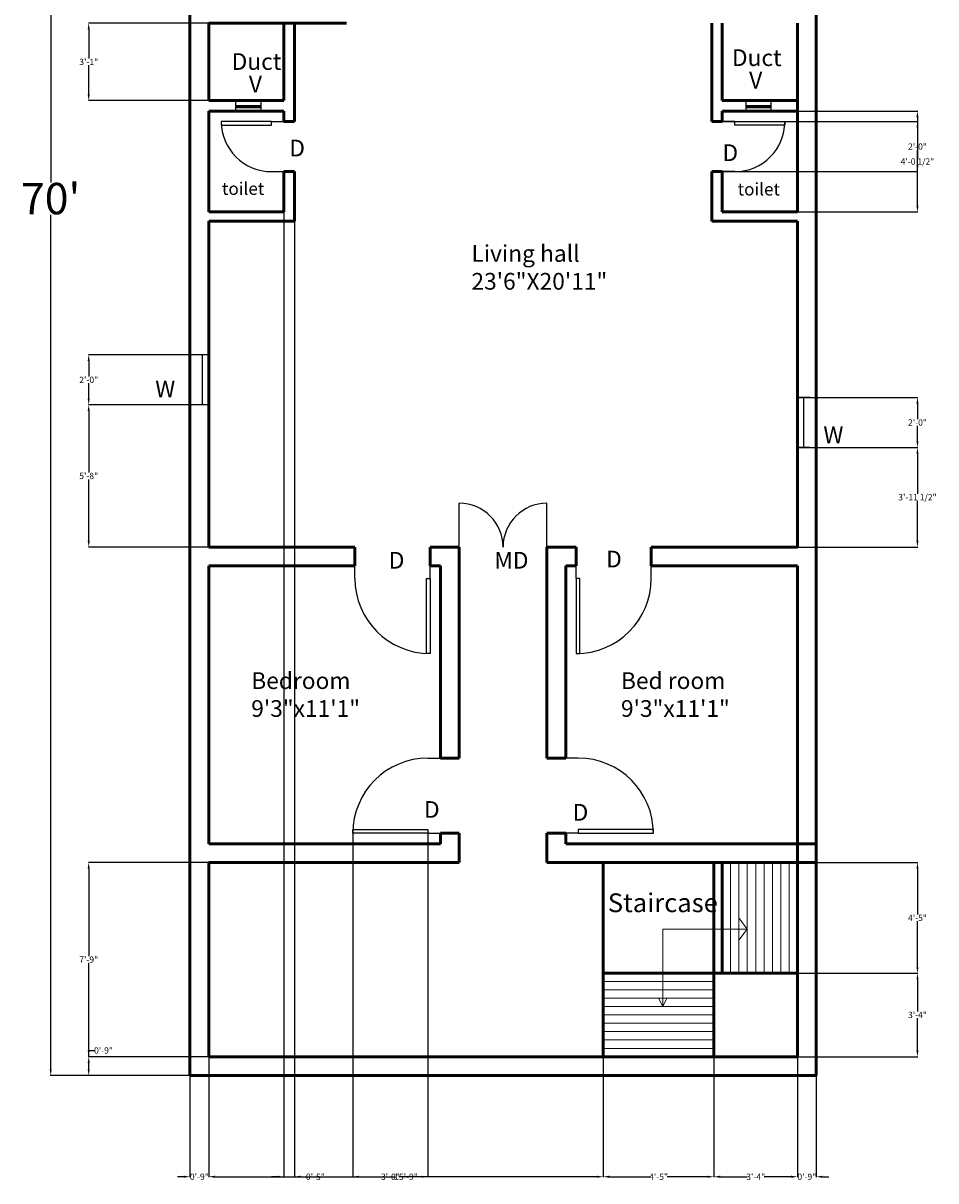
# Model space of a CAD drawing. Units: inches. Extents: x -250 to 2650, y 180 to 1183.
# Tile 9 of 10: x 2212 to 2650, y 180 to 734. Entities that reach past the tile are written whole.
import ezdxf

# ---------------------------------------------------------------- set-up
doc = ezdxf.new("R2010")
doc.units = ezdxf.units.IN
doc.header["$MEASUREMENT"] = 0
for name, color, linetype, lineweight in [('A-ANNO-DIMS', 2, 'Continuous', 18), ('A-ANNO-TEXT', 7, 'Continuous', 18), ('A-AREA-IDEN', 3, 'Continuous', 18), ('A-DOOR', 4, 'Continuous', 25), ('A-FLOR-STRS', 8, 'Continuous', 18), ('A-GLAZ', 3, 'Continuous', 25), ('A-WALL', 7, 'Continuous', 50)]:
    doc.layers.add(name, color=color, linetype=linetype, lineweight=lineweight)
doc.styles.get("Standard").update_dxf_attribs({"font": 'arial.ttf'})
doc.dimstyles.get("Standard").update_dxf_attribs({"dimtxt": 3, "dimasz": 3, "dimexe": 0.18, "dimexo": 0.0625, "dimgap": 0.09, "dimtad": 0, "dimtih": 1, "dimtoh": 1, "dimdec": 0, "dimzin": 0, "dimdsep": 46, "dimlunit": 3, "dimtxsty": 'Standard', "dimcen": 0.09, "dimadec": 0, "dimazin": 0, "dimtfac": 1, "dimtdec": 0, "dimtofl": 0, "dimtmove": 0, "dimatfit": 3, "dimfxl": 1, "dimtolj": 1, "dimtzin": 0, "dimarcsym": 0})

# ---------------------------------------------------------------- blocks, each defined once
blk = doc.blocks.new('*D39')
at = {"layer": 'A-ANNO-DIMS', "color": 0, "lineweight": -2, "transparency": 16777216}
for p, q in [((2292.12, 1070.02), (2225.3, 1070.02)), ((2225.48, 1067.02), (2225.48, 657.77)), ((2225.48, 233.02), (2225.48, 642.28)), ((2292.12, 230.02), (2225.3, 230.02))]:
    blk.add_line(p, q, dxfattribs=at)
at = {"layer": 'A-ANNO-DIMS', "color": 0, "transparency": 16777216}
for points in [[(2224.98, 1067.02), (2225.98, 1067.02), (2225.48, 1070.02)], [(2224.98, 233.02), (2225.98, 233.02), (2225.48, 230.02)]]:
    blk.add_solid(points, dxfattribs=at)
at = {"layer": 'Defpoints', "color": 0, "transparency": 16777216}
for p in [(2292.19, 1070.02), (2225.48, 230.02), (2292.19, 230.02)]:
    blk.add_point(p, dxfattribs=at)
at = {"layer": 'A-ANNO-DIMS', "color": 0, "transparency": 16777216, "insert": (2225.48, 650.02), "char_height": 3, "attachment_point": 5}
blk.add_mtext("\\A1;{\\H5x;70'}", dxfattribs=at)
blk = doc.blocks.new('*U27')
for p, q in [((0, 0), (0, -6)), ((24, 0), (24, -6))]:
    blk.add_line(p, q)
blk.add_lwpolyline([(0, 0), (0, 24), (1.75, 24), (1.75, 0)], close=True)
blk.add_arc((0, 0), 24, 0, 90)
blk = doc.blocks.new('*U28')
for p, q in [((0, 0), (0, 6)), ((24, 0), (24, 6))]:
    blk.add_line(p, q)
blk.add_lwpolyline([(0, 0), (0, -24), (1.75, -24), (1.75, 0)], close=True)
blk.add_arc((0, 0), 24, 270, 0)
blk = doc.blocks.new('*U29')
for p, q in [((0, 5), (0, 0)), ((0, 2.5), (12, 2.5)), ((12, 5), (12, 0))]:
    blk.add_line(p, q)
blk = doc.blocks.new('*U30')
for p, q in [((-36, 0), (-36, -6)), ((0, 0), (0, -6))]:
    blk.add_line(p, q)
blk.add_lwpolyline([(0, 0), (0, 36), (-1.75, 36), (-1.75, 0)], close=True)
blk.add_arc((0, 0), 36, 90, 180)
blk = doc.blocks.new('*U31')
for p, q in [((-36, 0), (-36, 6)), ((0, 0), (0, 6))]:
    blk.add_line(p, q)
blk.add_lwpolyline([(0, 0), (0, -36), (-1.75, -36), (-1.75, 0)], close=True)
blk.add_arc((0, 0), 36, 180, 270)
blk = doc.blocks.new('*U32')
for p, q in [((0, 0), (0, -6)), ((36, 0), (36, -6))]:
    blk.add_line(p, q)
blk.add_lwpolyline([(0, 0), (0, 36), (1.75, 36), (1.75, 0)], close=True)
blk.add_arc((0, 0), 36, 0, 90)
blk = doc.blocks.new('*U33')
for p, q in [((-36, 0), (-36, -6)), ((0, 0), (0, -6))]:
    blk.add_line(p, q)
blk.add_lwpolyline([(0, 0), (0, 36), (-1.75, 36), (-1.75, 0)], close=True)
blk.add_arc((0, 0), 36, 90, 180)
blk = doc.blocks.new('*U23')
for p, q in [((-24, 6), (-24, 0)), ((0, 6), (0, 0)), ((0, 3), (-24, 3))]:
    blk.add_line(p, q)
blk = doc.blocks.new('*U24')
for p, q in [((-24, 6), (-24, 0)), ((0, 6), (0, 0)), ((0, 3), (-24, 3))]:
    blk.add_line(p, q)
blk = doc.blocks.new('DOOR-DOUBLE-MAIN')
for p, q in [((505.08, 483.11), (505.08, 504.11)), ((505.08, 483.11), (505.08, 504.11)), ((547.08, 483.11), (547.08, 504.11))]:
    blk.add_line(p, q)
for centre, start, end in [((505.08, 483.11), 0, 90), ((505.08, 483.11), 0, 90), ((547.08, 483.11), 90, 180)]:
    blk.add_arc(centre, 21, start, end)
blk = doc.blocks.new('*D166')
at = {"layer": 'A-ANNO-DIMS', "color": 0, "lineweight": -2, "transparency": 16777216}
for p, q in [((2583.185258, 238.962048), (2583.185258, 181.344548)), ((2592.185258, 229.962048), (2592.185258, 181.344548)), ((2580.185258, 181.524548), (2577.185258, 181.524548)), ((2595.185258, 181.524548), (2598.185258, 181.524548))]:
    blk.add_line(p, q, dxfattribs=at)
at = {"layer": 'A-ANNO-DIMS', "color": 0, "transparency": 16777216}
for points in [[(2580.185258, 182.024548), (2580.185258, 181.024548), (2583.185258, 181.524548)], [(2595.185258, 182.024548), (2595.185258, 181.024548), (2592.185258, 181.524548)]]:
    blk.add_solid(points, dxfattribs=at)
at = {"layer": 'Defpoints', "color": 0, "transparency": 16777216}
for p in [(2583.185258, 239.024548), (2592.185258, 230.024548), (2592.185258, 181.524548)]:
    blk.add_point(p, dxfattribs=at)
at = {"layer": 'A-ANNO-DIMS', "color": 0, "transparency": 16777216, "insert": (2587.685258, 181.524548), "char_height": 3, "attachment_point": 5}
blk.add_mtext('\\A1;0\'-9"', dxfattribs=at)
blk = doc.blocks.new('*D167')
at = {"layer": 'A-ANNO-DIMS', "color": 0, "lineweight": -2, "transparency": 16777216}
for p, q in [((2301.185258, 238.962048), (2301.185258, 181.344548)), ((2292.185258, 229.962048), (2292.185258, 181.344548)), ((2289.185258, 181.524548), (2286.185258, 181.524548)), ((2304.185258, 181.524548), (2307.185258, 181.524548))]:
    blk.add_line(p, q, dxfattribs=at)
at = {"layer": 'A-ANNO-DIMS', "color": 0, "transparency": 16777216}
for points in [[(2289.185258, 182.024548), (2289.185258, 181.024548), (2292.185258, 181.524548)], [(2304.185258, 182.024548), (2304.185258, 181.024548), (2301.185258, 181.524548)]]:
    blk.add_solid(points, dxfattribs=at)
at = {"layer": 'Defpoints', "color": 0, "transparency": 16777216}
for p in [(2301.185258, 239.024548), (2292.185258, 230.024548), (2301.185258, 181.524548)]:
    blk.add_point(p, dxfattribs=at)
at = {"layer": 'A-ANNO-DIMS', "color": 0, "transparency": 16777216, "insert": (2296.685258, 181.524548), "char_height": 3, "attachment_point": 5}
blk.add_mtext('\\A1;0\'-9"', dxfattribs=at)
blk = doc.blocks.new('*D168')
at = {"layer": 'A-ANNO-DIMS', "color": 0, "lineweight": -2, "transparency": 16777216}
for p, q in [((2301.19, 238.96), (2301.19, 181.34)), ((2490.19, 238.96), (2490.19, 181.34)), ((2304.19, 181.52), (2390.58, 181.52)), ((2487.19, 181.52), (2400.79, 181.52))]:
    blk.add_line(p, q, dxfattribs=at)
at = {"layer": 'A-ANNO-DIMS', "color": 0, "transparency": 16777216}
for points in [[(2304.19, 182.02), (2304.19, 181.02), (2301.19, 181.52)], [(2487.19, 182.02), (2487.19, 181.02), (2490.19, 181.52)]]:
    blk.add_solid(points, dxfattribs=at)
at = {"layer": 'Defpoints', "color": 0, "transparency": 16777216}
for p in [(2301.19, 239.02), (2490.19, 239.02), (2490.19, 181.52)]:
    blk.add_point(p, dxfattribs=at)
at = {"layer": 'A-ANNO-DIMS', "color": 0, "transparency": 16777216, "insert": (2395.69, 181.52), "char_height": 3, "attachment_point": 5}
blk.add_mtext('\\A1;15\'-9"', dxfattribs=at)
blk = doc.blocks.new('*D169')
at = {"layer": 'A-ANNO-DIMS', "color": 0, "lineweight": -2, "transparency": 16777216}
for p, q in [((2490.19, 238.96), (2490.19, 181.34)), ((2543.19, 238.96), (2543.19, 181.34)), ((2493.19, 181.52), (2512.55, 181.52)), ((2540.19, 181.52), (2520.82, 181.52))]:
    blk.add_line(p, q, dxfattribs=at)
at = {"layer": 'A-ANNO-DIMS', "color": 0, "transparency": 16777216}
for points in [[(2493.19, 182.02), (2493.19, 181.02), (2490.19, 181.52)], [(2540.19, 182.02), (2540.19, 181.02), (2543.19, 181.52)]]:
    blk.add_solid(points, dxfattribs=at)
at = {"layer": 'Defpoints', "color": 0, "transparency": 16777216}
for p in [(2490.19, 239.02), (2543.19, 239.02), (2543.19, 181.52)]:
    blk.add_point(p, dxfattribs=at)
at = {"layer": 'A-ANNO-DIMS', "color": 0, "transparency": 16777216, "insert": (2516.69, 181.52), "char_height": 3, "attachment_point": 5}
blk.add_mtext('\\A1;4\'-5"', dxfattribs=at)
blk = doc.blocks.new('*D170')
at = {"layer": 'A-ANNO-DIMS', "color": 0, "lineweight": -2, "transparency": 16777216}
for p, q in [((2543.19, 238.96), (2543.19, 181.34)), ((2583.19, 238.96), (2583.19, 181.34)), ((2546.19, 181.52), (2559.11, 181.52)), ((2580.19, 181.52), (2567.26, 181.52))]:
    blk.add_line(p, q, dxfattribs=at)
at = {"layer": 'A-ANNO-DIMS', "color": 0, "transparency": 16777216}
for points in [[(2546.19, 182.02), (2546.19, 181.02), (2543.19, 181.52)], [(2580.19, 182.02), (2580.19, 181.02), (2583.19, 181.52)]]:
    blk.add_solid(points, dxfattribs=at)
at = {"layer": 'Defpoints', "color": 0, "transparency": 16777216}
for p in [(2543.19, 239.02), (2583.19, 239.02), (2583.19, 181.52)]:
    blk.add_point(p, dxfattribs=at)
at = {"layer": 'A-ANNO-DIMS', "color": 0, "transparency": 16777216, "insert": (2563.19, 181.52), "char_height": 3, "attachment_point": 5}
blk.add_mtext('\\A1;3\'-4"', dxfattribs=at)
blk = doc.blocks.new('*D171')
at = {"layer": 'A-ANNO-DIMS', "color": 0, "lineweight": -2, "transparency": 16777216}
for p, q in [((2583.25, 279.02), (2640.87, 279.02)), ((2640.69, 276.02), (2640.69, 260.65)), ((2640.69, 242.02), (2640.69, 257.4)), ((2583.25, 239.02), (2640.87, 239.02))]:
    blk.add_line(p, q, dxfattribs=at)
at = {"layer": 'A-ANNO-DIMS', "color": 0, "transparency": 16777216}
for points in [[(2640.19, 276.02), (2641.19, 276.02), (2640.69, 279.02)], [(2640.19, 242.02), (2641.19, 242.02), (2640.69, 239.02)]]:
    blk.add_solid(points, dxfattribs=at)
at = {"layer": 'Defpoints', "color": 0, "transparency": 16777216}
for p in [(2583.19, 279.02), (2640.69, 279.02), (2583.19, 239.02)]:
    blk.add_point(p, dxfattribs=at)
at = {"layer": 'A-ANNO-DIMS', "color": 0, "transparency": 16777216, "insert": (2640.69, 259.02), "char_height": 3, "attachment_point": 5}
blk.add_mtext('\\A1;3\'-4"', dxfattribs=at)
blk = doc.blocks.new('*D172')
at = {"layer": 'A-ANNO-DIMS', "color": 0, "lineweight": -2, "transparency": 16777216}
for p, q in [((2579.25, 332.02), (2640.87, 332.02)), ((2640.69, 329.02), (2640.69, 307.14)), ((2640.69, 282.02), (2640.69, 303.91)), ((2583.25, 279.02), (2640.87, 279.02))]:
    blk.add_line(p, q, dxfattribs=at)
at = {"layer": 'A-ANNO-DIMS', "color": 0, "transparency": 16777216}
for points in [[(2640.19, 329.02), (2641.19, 329.02), (2640.69, 332.02)], [(2640.19, 282.02), (2641.19, 282.02), (2640.69, 279.02)]]:
    blk.add_solid(points, dxfattribs=at)
at = {"layer": 'Defpoints', "color": 0, "transparency": 16777216}
for p in [(2579.19, 332.02), (2640.69, 332.02), (2583.19, 279.02)]:
    blk.add_point(p, dxfattribs=at)
at = {"layer": 'A-ANNO-DIMS', "color": 0, "transparency": 16777216, "insert": (2640.69, 305.52), "char_height": 3, "attachment_point": 5}
blk.add_mtext('\\A1;4\'-5"', dxfattribs=at)
blk = doc.blocks.new('*D173')
at = {"layer": 'A-ANNO-DIMS', "color": 0, "lineweight": -2, "transparency": 16777216}
for p, q in [((2301.12, 239.02), (2243.51, 239.02)), ((2243.69, 239.02), (2243.69, 242.02)), ((2243.69, 242.02), (2246.69, 242.02)), ((2243.69, 233.02), (2243.69, 236.02)), ((2292.12, 230.02), (2243.51, 230.02))]:
    blk.add_line(p, q, dxfattribs=at)
at = {"layer": 'A-ANNO-DIMS', "color": 0, "transparency": 16777216}
for points in [[(2243.19, 236.02), (2244.19, 236.02), (2243.69, 239.02)], [(2243.19, 233.02), (2244.19, 233.02), (2243.69, 230.02)]]:
    blk.add_solid(points, dxfattribs=at)
at = {"layer": 'Defpoints', "color": 0, "transparency": 16777216}
for p in [(2243.69, 239.02), (2301.19, 239.02), (2292.19, 230.02)]:
    blk.add_point(p, dxfattribs=at)
at = {"layer": 'A-ANNO-DIMS', "color": 0, "transparency": 16777216, "insert": (2250.76, 242.02), "char_height": 3, "attachment_point": 5}
blk.add_mtext('\\A1;0\'-9"', dxfattribs=at)
blk = doc.blocks.new('*D174')
at = {"layer": 'A-ANNO-DIMS', "color": 0, "lineweight": -2, "transparency": 16777216}
for p, q in [((2301.12, 332.02), (2243.51, 332.02)), ((2243.69, 329.02), (2243.69, 287.15)), ((2243.69, 242.02), (2243.69, 283.9)), ((2301.12, 239.02), (2243.51, 239.02))]:
    blk.add_line(p, q, dxfattribs=at)
at = {"layer": 'A-ANNO-DIMS', "color": 0, "transparency": 16777216}
for points in [[(2243.19, 329.02), (2244.19, 329.02), (2243.69, 332.02)], [(2243.19, 242.02), (2244.19, 242.02), (2243.69, 239.02)]]:
    blk.add_solid(points, dxfattribs=at)
at = {"layer": 'Defpoints', "color": 0, "transparency": 16777216}
for p in [(2243.69, 332.02), (2301.19, 332.02), (2301.19, 239.02)]:
    blk.add_point(p, dxfattribs=at)
at = {"layer": 'A-ANNO-DIMS', "color": 0, "transparency": 16777216, "insert": (2243.69, 285.52), "char_height": 3, "attachment_point": 5}
blk.add_mtext('\\A1;7\'-9"', dxfattribs=at)
blk = doc.blocks.new('*D176')
at = {"layer": 'A-ANNO-DIMS', "color": 0, "lineweight": -2, "transparency": 16777216}
for p, q in [((2337.19, 643.56), (2337.19, 181.34)), ((2342.19, 639.05), (2342.19, 181.34)), ((2334.19, 181.52), (2331.19, 181.52)), ((2345.19, 181.52), (2348.19, 181.52))]:
    blk.add_line(p, q, dxfattribs=at)
at = {"layer": 'A-ANNO-DIMS', "color": 0, "transparency": 16777216}
for points in [[(2334.19, 182.02), (2334.19, 181.02), (2337.19, 181.52)], [(2345.19, 182.02), (2345.19, 181.02), (2342.19, 181.52)]]:
    blk.add_solid(points, dxfattribs=at)
at = {"layer": 'Defpoints', "color": 0, "transparency": 16777216}
for p in [(2337.19, 643.62), (2342.19, 639.11), (2342.19, 181.52)]:
    blk.add_point(p, dxfattribs=at)
at = {"layer": 'A-ANNO-DIMS', "color": 0, "transparency": 16777216, "insert": (2352.26, 181.52), "char_height": 3, "attachment_point": 5}
blk.add_mtext('\\A1;0\'-5"', dxfattribs=at)
blk = doc.blocks.new('*D177')
at = {"layer": 'A-ANNO-DIMS', "color": 0, "lineweight": -2, "transparency": 16777216}
for p, q in [((2301.12, 734.02), (2243.51, 734.02)), ((2243.69, 731.02), (2243.69, 717.09)), ((2243.69, 699.91), (2243.69, 713.84)), ((2301.12, 696.91), (2243.51, 696.91))]:
    blk.add_line(p, q, dxfattribs=at)
at = {"layer": 'A-ANNO-DIMS', "color": 0, "transparency": 16777216}
for points in [[(2243.19, 731.02), (2244.19, 731.02), (2243.69, 734.02)], [(2243.19, 699.91), (2244.19, 699.91), (2243.69, 696.91)]]:
    blk.add_solid(points, dxfattribs=at)
at = {"layer": 'Defpoints', "color": 0, "transparency": 16777216}
for p in [(2243.69, 734.02), (2301.19, 734.02), (2301.19, 696.91)]:
    blk.add_point(p, dxfattribs=at)
at = {"layer": 'A-ANNO-DIMS', "color": 0, "transparency": 16777216, "insert": (2243.69, 715.47), "char_height": 3, "attachment_point": 5}
blk.add_mtext('\\A1;3\'-1"', dxfattribs=at)
blk = doc.blocks.new('*D178')
at = {"layer": 'A-ANNO-DIMS', "color": 0, "lineweight": -2, "transparency": 16777216}
for p, q in [((2583.25, 691.91), (2640.87, 691.91)), ((2640.69, 688.91), (2640.69, 669.41)), ((2640.69, 646.62), (2640.69, 666.12)), ((2583.25, 643.62), (2640.87, 643.62))]:
    blk.add_line(p, q, dxfattribs=at)
at = {"layer": 'A-ANNO-DIMS', "color": 0, "transparency": 16777216}
for points in [[(2640.19, 688.91), (2641.19, 688.91), (2640.69, 691.91)], [(2640.19, 646.62), (2641.19, 646.62), (2640.69, 643.62)]]:
    blk.add_solid(points, dxfattribs=at)
at = {"layer": 'Defpoints', "color": 0, "transparency": 16777216}
for p in [(2583.19, 691.91), (2640.69, 691.91), (2583.19, 643.62)]:
    blk.add_point(p, dxfattribs=at)
at = {"layer": 'A-ANNO-DIMS', "color": 0, "transparency": 16777216, "insert": (2640.69, 667.77), "char_height": 3, "attachment_point": 5}
blk.add_mtext('\\A1;4\'-0 1/2"', dxfattribs=at)
blk = doc.blocks.new('*D179')
at = {"layer": 'A-ANNO-DIMS', "color": 0, "lineweight": -2, "transparency": 16777216}
for p, q in [((2583.25, 530.79), (2640.87, 530.79)), ((2640.69, 527.79), (2640.69, 508.59)), ((2640.69, 486.11), (2640.69, 505.31)), ((2583.25, 483.11), (2640.87, 483.11))]:
    blk.add_line(p, q, dxfattribs=at)
at = {"layer": 'A-ANNO-DIMS', "color": 0, "transparency": 16777216}
for points in [[(2640.19, 527.79), (2641.19, 527.79), (2640.69, 530.79)], [(2640.19, 486.11), (2641.19, 486.11), (2640.69, 483.11)]]:
    blk.add_solid(points, dxfattribs=at)
at = {"layer": 'Defpoints', "color": 0, "transparency": 16777216}
for p in [(2583.19, 530.79), (2640.69, 530.79), (2583.19, 483.11)]:
    blk.add_point(p, dxfattribs=at)
at = {"layer": 'A-ANNO-DIMS', "color": 0, "transparency": 16777216, "insert": (2640.69, 506.95), "char_height": 3, "attachment_point": 5}
blk.add_mtext('\\A1;3\'-11 1/2"', dxfattribs=at)
blk = doc.blocks.new('*D180')
at = {"layer": 'A-ANNO-DIMS', "color": 0, "lineweight": -2, "transparency": 16777216}
for p, q in [((2583.25, 554.79), (2640.87, 554.79)), ((2640.69, 551.79), (2640.69, 544.41)), ((2640.69, 533.79), (2640.69, 541.16)), ((2583.25, 530.79), (2640.87, 530.79))]:
    blk.add_line(p, q, dxfattribs=at)
at = {"layer": 'A-ANNO-DIMS', "color": 0, "transparency": 16777216}
for points in [[(2640.19, 551.79), (2641.19, 551.79), (2640.69, 554.79)], [(2640.19, 533.79), (2641.19, 533.79), (2640.69, 530.79)]]:
    blk.add_solid(points, dxfattribs=at)
at = {"layer": 'Defpoints', "color": 0, "transparency": 16777216}
for p in [(2583.19, 554.79), (2640.69, 554.79), (2583.19, 530.79)]:
    blk.add_point(p, dxfattribs=at)
at = {"layer": 'A-ANNO-DIMS', "color": 0, "transparency": 16777216, "insert": (2640.69, 542.79), "char_height": 3, "attachment_point": 5}
blk.add_mtext('\\A1;2\'-0"', dxfattribs=at)
blk = doc.blocks.new('*D181')
at = {"layer": 'A-ANNO-DIMS', "color": 0, "lineweight": -2, "transparency": 16777216}
for p, q in [((2301.12, 551.2), (2243.51, 551.2)), ((2243.69, 548.2), (2243.69, 518.78)), ((2243.69, 486.11), (2243.69, 515.53)), ((2301.12, 483.11), (2243.51, 483.11))]:
    blk.add_line(p, q, dxfattribs=at)
at = {"layer": 'A-ANNO-DIMS', "color": 0, "transparency": 16777216}
for points in [[(2243.19, 548.2), (2244.19, 548.2), (2243.69, 551.2)], [(2243.19, 486.11), (2244.19, 486.11), (2243.69, 483.11)]]:
    blk.add_solid(points, dxfattribs=at)
at = {"layer": 'Defpoints', "color": 0, "transparency": 16777216}
for p in [(2243.69, 551.2), (2301.19, 551.2), (2301.19, 483.11)]:
    blk.add_point(p, dxfattribs=at)
at = {"layer": 'A-ANNO-DIMS', "color": 0, "transparency": 16777216, "insert": (2243.69, 517.16), "char_height": 3, "attachment_point": 5}
blk.add_mtext('\\A1;5\'-8"', dxfattribs=at)
blk = doc.blocks.new('*D182')
at = {"layer": 'A-ANNO-DIMS', "color": 0, "lineweight": -2, "transparency": 16777216}
for p, q in [((2301.12, 575.2), (2243.51, 575.2)), ((2243.69, 572.2), (2243.69, 564.82)), ((2243.69, 554.2), (2243.69, 561.58)), ((2301.12, 551.2), (2243.51, 551.2))]:
    blk.add_line(p, q, dxfattribs=at)
at = {"layer": 'A-ANNO-DIMS', "color": 0, "transparency": 16777216}
for points in [[(2243.19, 572.2), (2244.19, 572.2), (2243.69, 575.2)], [(2243.19, 554.2), (2244.19, 554.2), (2243.69, 551.2)]]:
    blk.add_solid(points, dxfattribs=at)
at = {"layer": 'Defpoints', "color": 0, "transparency": 16777216}
for p in [(2243.69, 575.2), (2301.19, 575.2), (2301.19, 551.2)]:
    blk.add_point(p, dxfattribs=at)
at = {"layer": 'A-ANNO-DIMS', "color": 0, "transparency": 16777216, "insert": (2243.69, 563.2), "char_height": 3, "attachment_point": 5}
blk.add_mtext('\\A1;2\'-0"', dxfattribs=at)
blk = doc.blocks.new('*D183')
at = {"layer": 'A-ANNO-DIMS', "color": 0, "lineweight": -2, "transparency": 16777216}
for p, q in [((2370.19, 345.96), (2370.19, 181.34)), ((2406.19, 345.96), (2406.19, 181.34)), ((2373.19, 181.52), (2384.11, 181.52)), ((2403.19, 181.52), (2392.26, 181.52))]:
    blk.add_line(p, q, dxfattribs=at)
at = {"layer": 'A-ANNO-DIMS', "color": 0, "transparency": 16777216}
for points in [[(2373.19, 182.02), (2373.19, 181.02), (2370.19, 181.52)], [(2403.19, 182.02), (2403.19, 181.02), (2406.19, 181.52)]]:
    blk.add_solid(points, dxfattribs=at)
at = {"layer": 'Defpoints', "color": 0, "transparency": 16777216}
for p in [(2370.19, 346.02), (2406.19, 346.02), (2406.19, 181.52)]:
    blk.add_point(p, dxfattribs=at)
at = {"layer": 'A-ANNO-DIMS', "color": 0, "transparency": 16777216, "insert": (2388.19, 181.52), "char_height": 3, "attachment_point": 5}
blk.add_mtext('\\A1;3\'-0"', dxfattribs=at)
blk = doc.blocks.new('*D184')
at = {"layer": 'A-ANNO-DIMS', "color": 0, "lineweight": -2, "transparency": 16777216}
for p, q in [((2542.25, 686.91), (2640.87, 686.91)), ((2640.69, 683.91), (2640.69, 676.53)), ((2640.69, 665.91), (2640.69, 673.29)), ((2542.25, 662.91), (2640.87, 662.91))]:
    blk.add_line(p, q, dxfattribs=at)
at = {"layer": 'A-ANNO-DIMS', "color": 0, "transparency": 16777216}
for points in [[(2640.19, 683.91), (2641.19, 683.91), (2640.69, 686.91)], [(2640.19, 665.91), (2641.19, 665.91), (2640.69, 662.91)]]:
    blk.add_solid(points, dxfattribs=at)
at = {"layer": 'Defpoints', "color": 0, "transparency": 16777216}
for p in [(2542.19, 686.91), (2640.69, 686.91), (2542.19, 662.91)]:
    blk.add_point(p, dxfattribs=at)
at = {"layer": 'A-ANNO-DIMS', "color": 0, "transparency": 16777216, "insert": (2640.69, 674.91), "char_height": 3, "attachment_point": 5}
blk.add_mtext('\\A1;2\'-0"', dxfattribs=at)

msp = doc.modelspace()

# ---------------------------------------------------------------- linework, layer by layer
at = {"layer": 'A-FLOR-STRS'}
for p, q in [((2551.19, 279.02), (2551.19, 332.02)), ((2555.19, 279.02), (2555.19, 332.02)), ((2559.19, 279.02), (2559.19, 332.02)), ((2563.19, 279.02), (2563.19, 332.02)), ((2567.19, 279.02), (2567.19, 332.02)), ((2571.19, 279.02), (2571.19, 332.02)), ((2575.19, 279.02), (2575.19, 332.02)), ((2579.19, 279.02), (2579.19, 332.02)), ((2559.19, 300.14), (2555.19, 305.52)), ((2518.7, 300.14), (2518.7, 263.02)), ((2518.7, 300.14), (2559.19, 300.14)), ((2559.19, 300.14), (2555.19, 294.75)), ((2490.19, 275.02), (2543.19, 275.02)), ((2490.19, 271.02), (2543.19, 271.02)), ((2490.19, 267.02), (2543.19, 267.02)), ((2518.7, 263.02), (2516.69, 267.02)), ((2518.7, 263.02), (2520.71, 267.02)), ((2490.19, 263.02), (2543.19, 263.02)), ((2490.19, 259.02), (2543.19, 259.02)), ((2490.19, 255.02), (2543.19, 255.02)), ((2490.19, 251.02), (2543.19, 251.02)), ((2490.19, 247.02), (2543.19, 247.02)), ((2490.19, 243.02), (2543.19, 243.02))]:
    msp.add_line(p, q, dxfattribs=at)
at = {"layer": 'A-WALL'}
for p, q in [((2292.19, 1070.02), (2292.19, 230.02)), ((2592.19, 230.02), (2592.19, 1070.02)), ((2367.19, 734.02), (2301.19, 734.02)), ((2301.19, 734.02), (2301.19, 696.91)), ((2337.19, 696.91), (2337.19, 734.02)), ((2342.19, 686.91), (2342.19, 734.02)), ((2542.19, 686.91), (2542.19, 734.02)), ((2542.19, 686.91), (2542.19, 734.02)), ((2547.19, 696.91), (2547.19, 734.02)), ((2583.19, 643.62), (2583.19, 734.02)), ((2583.19, 696.91), (2583.19, 734.02)), ((2583.19, 716.02), (2583.19, 734.02)), ((2337.19, 696.91), (2301.19, 696.91)), ((2326.24, 693.93), (2314.24, 693.93)), ((2583.19, 696.91), (2547.19, 696.91)), ((2570.63, 693.93), (2558.63, 693.93)), ((2301.19, 691.91), (2301.19, 643.62)), ((2337.19, 691.91), (2301.19, 691.91)), ((2337.19, 691.91), (2337.19, 686.91)), ((2547.19, 686.91), (2547.19, 691.91)), ((2583.19, 691.91), (2547.19, 691.91)), ((2583.19, 643.62), (2583.19, 691.91)), ((2337.19, 686.91), (2342.19, 686.91)), ((2547.19, 686.91), (2542.19, 686.91)), ((2337.19, 662.91), (2337.19, 643.62)), ((2337.19, 662.91), (2342.19, 662.91)), ((2342.19, 639.11), (2342.19, 662.91)), ((2342.19, 662.91), (2342.19, 639.11)), ((2542.19, 639.11), (2542.19, 662.91)), ((2542.19, 643.62), (2542.19, 662.91)), ((2547.19, 662.91), (2542.19, 662.91)), ((2547.19, 643.62), (2547.19, 662.91)), ((2337.19, 643.62), (2301.19, 643.62)), ((2342.19, 643.62), (2342.19, 643.62)), ((2583.19, 643.62), (2547.19, 643.62)), ((2301.19, 639.11), (2301.19, 483.11)), ((2342.19, 639.11), (2301.19, 639.11)), ((2583.19, 639.11), (2542.19, 639.11)), ((2583.19, 483.11), (2583.19, 639.11)), ((2583.19, 587.02), (2583.19, 639.11)), ((2371.19, 483.11), (2301.19, 483.11)), ((2371.19, 474.11), (2371.19, 483.11)), ((2421.19, 483.11), (2407.19, 483.11)), ((2407.19, 474.11), (2407.19, 483.11)), ((2421.19, 483.11), (2421.19, 382.02)), ((2463.19, 382.02), (2463.19, 483.11)), ((2477.19, 483.11), (2463.19, 483.11)), ((2477.19, 474.11), (2477.19, 483.11)), ((2583.19, 483.11), (2513.19, 483.11)), ((2513.19, 474.11), (2513.19, 483.11)), ((2301.19, 474.11), (2301.19, 341.02)), ((2371.19, 474.11), (2301.19, 474.11)), ((2412.19, 474.11), (2407.19, 474.11)), ((2412.19, 474.11), (2412.19, 382.02)), ((2472.19, 382.02), (2472.19, 474.11)), ((2477.19, 474.11), (2472.19, 474.11)), ((2583.19, 474.11), (2513.19, 474.11)), ((2583.19, 239.02), (2583.19, 474.11)), ((2412.19, 382.02), (2421.19, 382.02)), ((2463.19, 382.02), (2472.19, 382.02)), ((2412.19, 346.02), (2412.19, 341.02)), ((2412.19, 346.02), (2421.19, 346.02)), ((2421.19, 346.02), (2421.19, 332.02)), ((2463.19, 332.02), (2463.19, 346.02)), ((2472.19, 346.02), (2463.19, 346.02)), ((2472.19, 341.02), (2472.19, 346.02)), ((2301.19, 341.02), (2412.19, 341.02)), ((2472.19, 341.02), (2592.19, 341.02)), ((2301.19, 332.02), (2421.19, 332.02)), ((2301.19, 332.02), (2301.19, 239.02)), ((2463.19, 332.02), (2592.19, 332.02)), ((2490.19, 239.02), (2490.19, 332.02)), ((2543.19, 239.02), (2543.19, 332.02)), ((2547.19, 279.02), (2547.19, 332.02)), ((2490.19, 279.02), (2583.19, 279.02)), ((2301.19, 239.02), (2325.94, 239.02)), ((2301.19, 239.02), (2583.19, 239.02)), ((2292.19, 230.02), (2325.19, 230.02)), ((2292.19, 230.02), (2592.19, 230.02))]:
    msp.add_line(p, q, dxfattribs=at)

# ---------------------------------------------------------------- block references
at = {"layer": 'A-DOOR'}
for name, p, rotation in [('*U28', (2331.19, 686.91), 270), ('*U27', (2553.19, 686.91), 270), ('*U32', (2407.19, 468.11), 180), ('*U33', (2477.19, 468.11), 180), ('*U31', (2406.19, 346.02), 270), ('*U30', (2478.19, 346.02), 270)]:
    msp.add_blockref(name, p, dxfattribs=dict(at, rotation=rotation))
msp.add_blockref('DOOR-DOUBLE-MAIN', (1916.1, 0), dxfattribs=at)
at = {"layer": 'A-GLAZ'}
for name, p, rotation in [('*U29', (2326.24, 696.91), 180), ('*U29', (2570.63, 696.91), 180), ('*U23', (2295.19, 551.2), 270), ('*U24', (2583.19, 530.79), 270)]:
    msp.add_blockref(name, p, dxfattribs=dict(at, rotation=rotation))

# ---------------------------------------------------------------- texts
at = {"layer": 'A-ANNO-TEXT', "char_height": 8, "attachment_point": 1}
for s, insert in [('V', (2560.06, 710.71)), ('V', (2320.41, 708.86)), ('D', (2339.77, 678.19)), ('D', (2547.27, 675.98)), ('W', (2275.55, 562.85)), ('W', (2595.62, 540.86)), ('D', (2387.42, 480.78)), ('MD', (2437.99, 480.78)), ('D', (2491.54, 481.35)), ('D', (2404.29, 361.42)), ('D', (2475.5, 360.07))]:
    msp.add_mtext_dynamic_manual_height_columns(s, width=10.3916, gutter_width=1, heights=[0], dxfattribs=dict(at, insert=insert))
at = {"layer": 'A-AREA-IDEN', "attachment_point": 1}
for s, width, heights, insert, char_height in [('{\\H2.66667x;Duct} ', 7.71, [3.05], (2551.8, 721.49), 3), ('{\\H2.66667x;Duct} ', 7.71, [3.05], (2312.15, 719.65), 3), ('toilet', 19.3499, [0], (2307.53, 657.78), 6), ('toilet', 19.3499, [0], (2554.57, 657.5), 6), ('Living hall  \\P23\'6"X20\'11"', 123.5412, [0], (2427.03, 627.72), 8), ('Bedroom 9\'3"x11\'1"', 88.0689, [0], (2321.54, 423.12), 8), ('Bed room 9\'3"x11\'1"', 88.0689, [0], (2498.66, 423.12), 8), ('Staircase  ', 87.4783, [0], (2492.36, 317.24), 9)]:
    msp.add_mtext_dynamic_manual_height_columns(s, width=width, gutter_width=1, heights=heights, dxfattribs=dict(at, insert=insert, char_height=char_height))

# ---------------------------------------------------------------- dimensions: what is measured, and where the dimension line sits
at = {"layer": 'A-ANNO-DIMS'}
dim = msp.add_linear_dim(base=(2225.48, 230.02), p1=(2292.19, 1070.02), p2=(2292.19, 230.02), angle=90, text='{\\H5x;<>}', dimstyle='Standard', override={"dimclrd": 0, "dimclre": 0, "dimclrt": 0}, dxfattribs=at)
dim.commit()
dim.dimension.update_dxf_attribs({"geometry": '*D39', "text_midpoint": (2225.48, 650.02)})
for base, p1, p2, picture, middle in [((2243.69, 734.02), (2301.19, 696.91), (2301.19, 734.02), '*D177', (2243.69, 715.47)), ((2640.69, 691.91), (2583.19, 643.62), (2583.19, 691.91), '*D178', (2640.69, 667.77)), ((2640.69, 686.91), (2542.19, 662.91), (2542.19, 686.91), '*D184', (2640.69, 674.91)), ((2243.69, 575.2), (2301.19, 551.2), (2301.19, 575.2), '*D182', (2243.69, 563.2)), ((2640.69, 554.79), (2583.19, 530.79), (2583.19, 554.79), '*D180', (2640.69, 542.79)), ((2243.69, 551.2), (2301.19, 483.11), (2301.19, 551.2), '*D181', (2243.69, 517.16)), ((2640.69, 530.79), (2583.19, 483.11), (2583.19, 530.79), '*D179', (2640.69, 506.95)), ((2243.69, 332.02), (2301.19, 239.02), (2301.19, 332.02), '*D174', (2243.69, 285.52)), ((2640.69, 332.02), (2583.19, 279.02), (2579.19, 332.02), '*D172', (2640.69, 305.52)), ((2640.69, 279.02), (2583.19, 239.02), (2583.19, 279.02), '*D171', (2640.69, 259.02)), ((2243.69, 239.02), (2292.19, 230.02), (2301.19, 239.02), '*D173', (2250.76, 242.02))]:
    dim = msp.add_linear_dim(base=base, p1=p1, p2=p2, angle=90, dimstyle='Standard', override={"dimdec": 1, "dimlfac": 1, "dimrnd": 0, "dimzin": 1, "dimdsep": 46, "dimlunit": 4, "dimfrac": 2}, dxfattribs=at)
    dim.commit()
    dim.dimension.update_dxf_attribs({"geometry": picture, "text_midpoint": middle})
for base, p1, p2, picture, middle in [((2342.19, 181.52), (2337.19, 643.62), (2342.19, 639.11), '*D176', (2352.26, 181.52)), ((2406.19, 181.52), (2370.19, 346.02), (2406.19, 346.02), '*D183', (2388.19, 181.52)), ((2301.19, 181.52), (2292.19, 230.02), (2301.19, 239.02), '*D167', (2296.69, 181.52)), ((2490.19, 181.52), (2301.19, 239.02), (2490.19, 239.02), '*D168', (2395.69, 181.52)), ((2543.19, 181.52), (2490.19, 239.02), (2543.19, 239.02), '*D169', (2516.69, 181.52)), ((2583.19, 181.52), (2543.19, 239.02), (2583.19, 239.02), '*D170', (2563.19, 181.52)), ((2592.19, 181.52), (2583.19, 239.02), (2592.19, 230.02), '*D166', (2587.69, 181.52))]:
    dim = msp.add_linear_dim(base=base, p1=p1, p2=p2, dimstyle='Standard', override={"dimdec": 1, "dimlfac": 1, "dimrnd": 0, "dimzin": 1, "dimdsep": 46, "dimlunit": 4, "dimfrac": 2}, dxfattribs=at)
    dim.commit()
    dim.dimension.update_dxf_attribs({"geometry": picture, "text_midpoint": middle})

doc.saveas('drawing.dxf')
